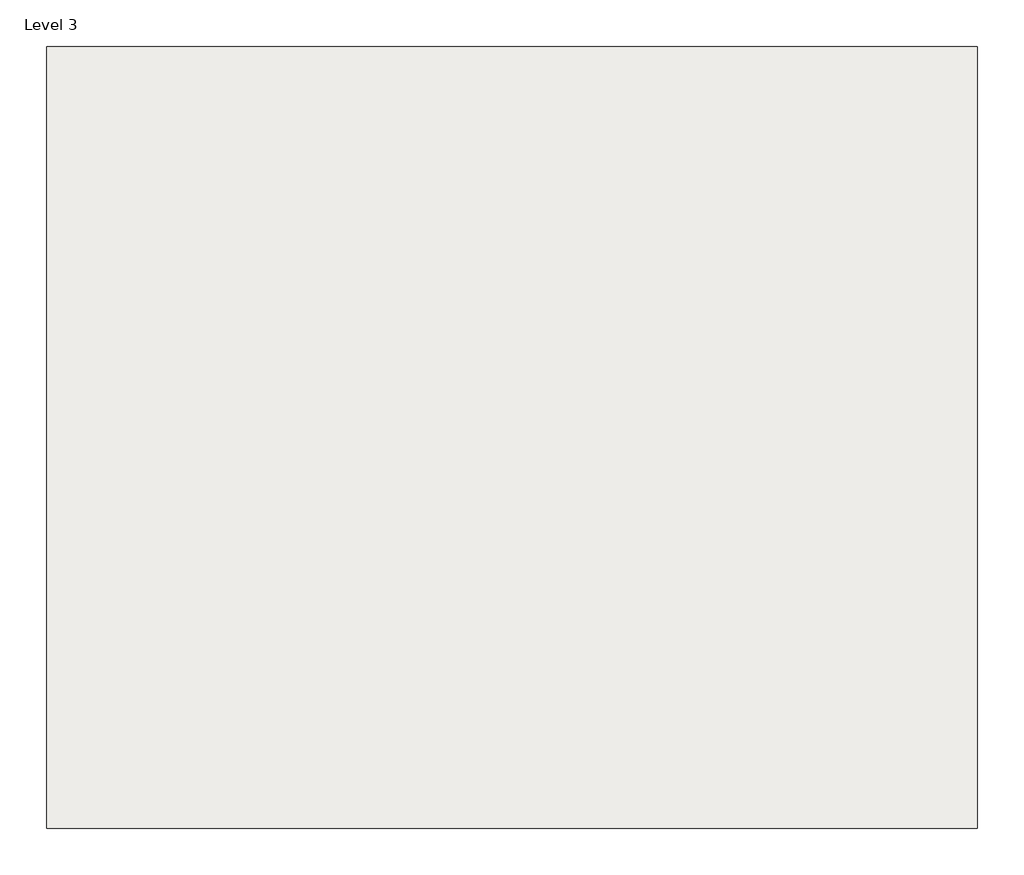
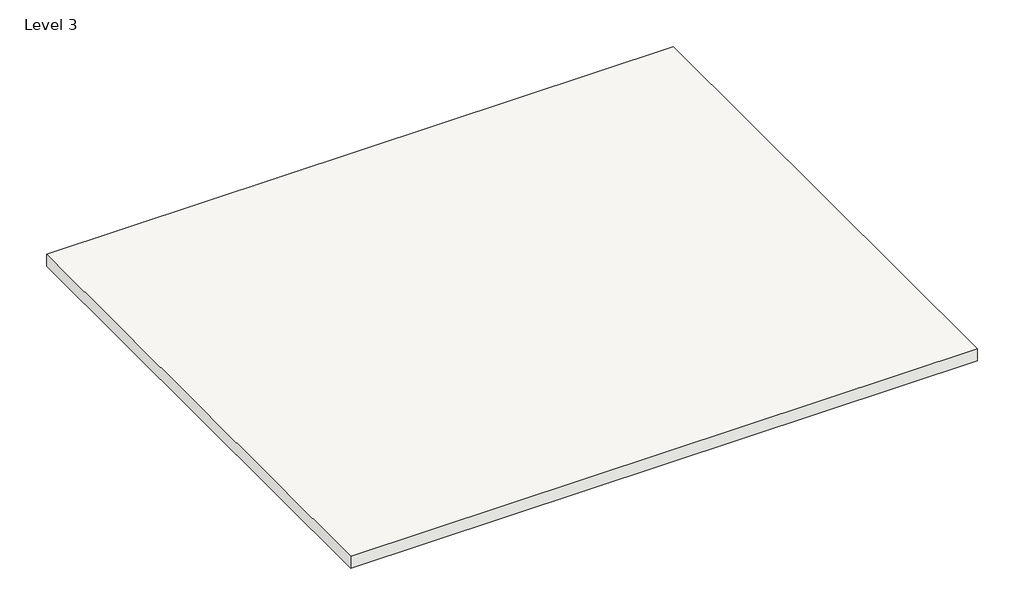
# One storey: 1 roof.
"""IFC4 building model written with IfcOpenShell, lengths in millimetres."""

from ifc_helpers import new_model, si_unit, frame, origin, place, context, project, spatial, polyline, outline, extrude, element, save

model = new_model("IFC4")

# Units and contexts
model_context = context("Model", 3, world=origin())
ifc_project = project(units=[si_unit("LENGTHUNIT", "METRE", prefix="MILLI")], contexts=[model_context])

# Site, building, storey
site = spatial("IfcSite", under=ifc_project)
building = spatial("IfcBuilding", under=site)
storey = spatial("IfcBuildingStorey", under=building, Name="Level 3", Elevation=6096.0)

# Roof
placement = place(None, origin())
element("IfcRoof", 1, ObjectType="Generic - 12\"", at=placement, inside=storey, context=model_context, shape_type="SweptSolid", body=[
    extrude(outline(polyline([(-17842.4229687, 1630.8984882), (-2983.4229687, 1630.8984882), (-2983.4229687, -10853.2015118), (-17842.4229687, -10853.2015118), (-17842.4229687, 1630.8984882)])), frame((0.0, 0.0, 6096.0), z_axis=(0.0, 0.0, 1.0), x_axis=(1.0, 0.0, 0.0)), (0.0, 0.0, 1.0), 304.8),
])

save(model, "model.ifc")

# Revit data of these elements
# Type "Generic - 12\""
#   Assembly Code = "B1020"
#   Layers, outside or top first: 1' - 0" no material (function 1)
# Element 1 (IfcRoof, "Generic - 12\"")
#   built-in parameter 1001705 = 21 (stored number, unit not read)
#   built-in parameter 1001710 = 33615
#   Phase Created = New Construction
#   Materials on its faces: "Default Roof"
# Materials
#   "Default Roof": colour RGB 88 101 114, transparency 0, Cost = 0
